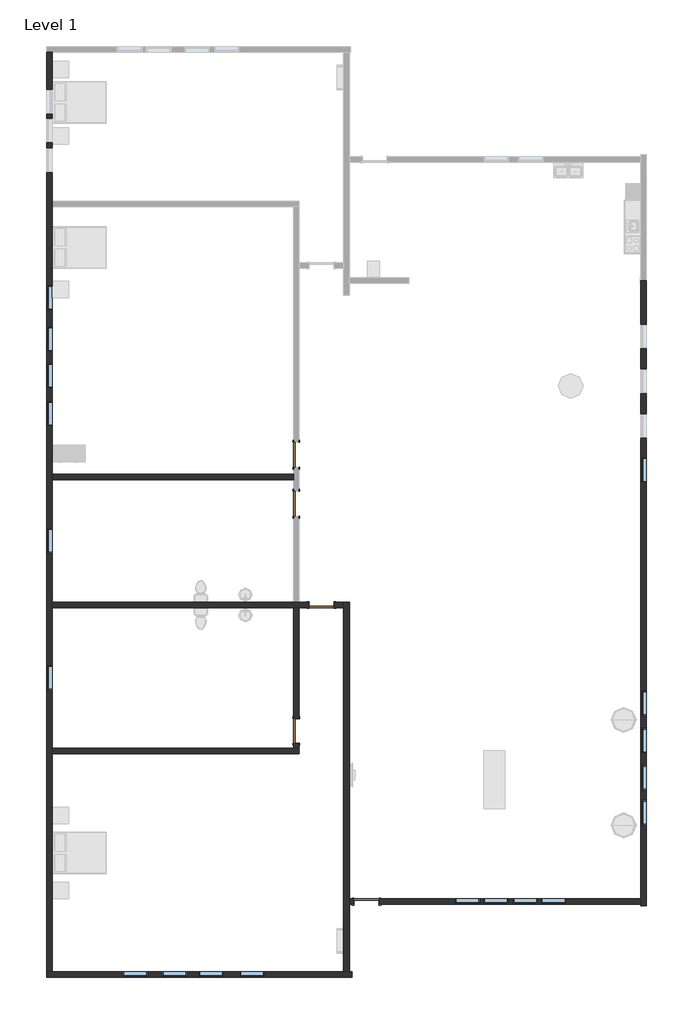
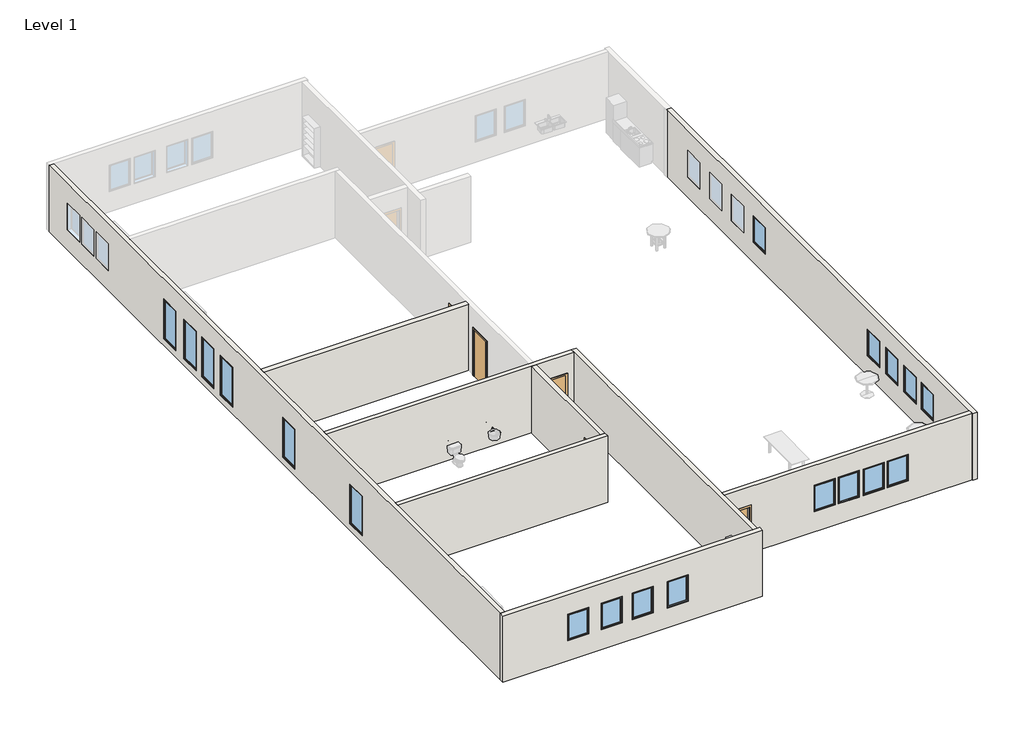
# One storey, part 1 of 2: 19 windows, 9 walls, 5 doors.
"""IFC4 building model written with IfcOpenShell, lengths in millimetres."""

from ifc_helpers import new_model, si_unit, frame, origin, origin_with_axes, place, context, project, spatial, polyline, outline, extrude, faceted_brep, transform, mapped, element, save
from components import door_54dd4da4, door_719f80de, window_e2841890, window_9a779fa2

model = new_model("IFC4")

# Units and contexts
model_context = context("Model", 3, world=origin())
ifc_project = project(units=[si_unit("LENGTHUNIT", "METRE", prefix="MILLI")], contexts=[model_context])

# Site, building, storey
site = spatial("IfcSite", under=ifc_project)
building = spatial("IfcBuilding", under=site)
storey = spatial("IfcBuildingStorey", under=building, Name="Level 1", Elevation=0.0)

# Doors
placement = place(None, origin())
door_shape = door_54dd4da4(model_context)
element("IfcDoor", 1, ObjectType="Single-Flush : 36\" x 84\"", at=placement, inside=storey, context=model_context, shape_type="MappedRepresentation", body=[
    mapped(door_shape, transform((-5497.7112155, -2495.646371, 0.0), x_axis=(0.0, 1.0, 0.0), y_axis=(-1.0, 0.0, 0.0), z_axis=(0.0, 0.0, 1.0))),
])
door_2_shape = door_719f80de(model_context)
element("IfcDoor", 2, ObjectType="Single-Flush : 36\" x 84\"", at=placement, inside=storey, context=model_context, shape_type="MappedRepresentation", body=[
    mapped(door_2_shape, transform((-4570.6112155, -6229.446371, 0.0), x_axis=(1.0, 0.0, 0.0), y_axis=(0.0, 1.0, 0.0), z_axis=(0.0, 0.0, 1.0))),
])
element("IfcDoor", 3, ObjectType="Single-Flush : 36\" x 84\"", at=placement, inside=storey, context=model_context, shape_type="MappedRepresentation", body=[
    mapped(door_2_shape, transform((-5497.7112155, -10877.646371, 0.0), x_axis=(0.0, -1.0, 0.0), y_axis=(1.0, 0.0, 0.0), z_axis=(0.0, 0.0, 1.0))),
])
element("IfcDoor", 4, ObjectType="Single-Flush : 36\" x 84\"", at=placement, inside=storey, context=model_context, shape_type="MappedRepresentation", body=[
    mapped(door_2_shape, transform((-2906.9112155, -17176.846371, 0.0), x_axis=(-1.0, 0.0, 0.0), y_axis=(0.0, -1.0, 0.0), z_axis=(0.0, 0.0, 1.0))),
])
element("IfcDoor", 5, ObjectType="Single-Flush : 36\" x 84\"", at=placement, inside=storey, context=model_context, shape_type="MappedRepresentation", body=[
    mapped(door_2_shape, transform((-5497.7112155, -692.246371, 0.0), x_axis=(0.0, -1.0, 0.0), y_axis=(1.0, 0.0, 0.0), z_axis=(0.0, 0.0, 1.0))),
])

# Walls
element("IfcWall", 6, ObjectType="Generic - 8\"", at=placement, inside=storey, context=model_context, shape_type="Brep", body=[
    faceted_brep([(-14514.7112155, -19767.646371, 0.0), (-14514.7112155, -11715.846371, 0.0), (-14514.7112155, -11512.646371, 0.0), (-14514.7112155, -6331.046371, 0.0), (-14514.7112155, -6127.846371, 0.0), (-14514.7112155, -1606.646371, 0.0), (-14514.7112155, -1403.446371, 0.0), (-14514.7112155, 8451.753629, 0.0), (-14514.7112155, 8654.953629, 0.0), (-14514.7112155, 14166.753629, 0.0), (-14514.7112155, 14166.753629, 3048.0), (-14514.7112155, 8654.953629, 3048.0), (-14514.7112155, 8451.753629, 3048.0), (-14514.7112155, -1403.446371, 3048.0), (-14514.7112155, -1606.646371, 3048.0), (-14514.7112155, -6127.846371, 3048.0), (-14514.7112155, -6331.046371, 3048.0), (-14514.7112155, -11512.646371, 3048.0), (-14514.7112155, -11715.846371, 3048.0), (-14514.7112155, -19767.646371, 3048.0), (-14514.7112155, 11880.753629, 2133.6), (-14514.7112155, 12795.153629, 2133.6), (-14514.7112155, 12795.153629, 914.4), (-14514.7112155, 11880.753629, 914.4), (-14514.7112155, 11728.353629, 2133.6), (-14514.7112155, 11728.353629, 914.4), (-14514.7112155, 10813.953629, 914.4), (-14514.7112155, 10813.953629, 2133.6), (-14514.7112155, 10636.153629, 2133.6), (-14514.7112155, 10636.153629, 914.4), (-14514.7112155, 9721.753629, 914.4), (-14514.7112155, 9721.753629, 2133.6), (-14514.7112155, -8464.646371, 2133.6), (-14514.7112155, -8464.646371, 304.8), (-14514.7112155, -9379.046371, 304.8), (-14514.7112155, -9379.046371, 2133.6), (-14514.7112155, -3410.046371, 2133.6), (-14514.7112155, -3410.046371, 304.8), (-14514.7112155, -4324.446371, 304.8), (-14514.7112155, -4324.446371, 2133.6), (-14514.7112155, 1288.953629, 2133.6), (-14514.7112155, 1288.953629, 304.8), (-14514.7112155, 374.553629, 304.8), (-14514.7112155, 374.553629, 2133.6), (-14514.7112155, 2685.953629, 2133.6), (-14514.7112155, 2685.953629, 304.8), (-14514.7112155, 1771.553629, 304.8), (-14514.7112155, 1771.553629, 2133.6), (-14514.7112155, 4032.153629, 2133.6), (-14514.7112155, 4032.153629, 304.8), (-14514.7112155, 3117.753629, 304.8), (-14514.7112155, 3117.753629, 2133.6), (-14514.7112155, 5556.153629, 2133.6), (-14514.7112155, 5556.153629, 304.8), (-14514.7112155, 4641.753629, 304.8), (-14514.7112155, 4641.753629, 2133.6), (-14717.9112155, -19767.646371, 0.0), (-14717.9112155, -19767.646371, 3048.0), (-14717.9112155, 14166.753629, 3048.0), (-14717.9112155, 14166.753629, 0.0), (-14717.9112155, 11880.753629, 2133.6), (-14717.9112155, 11880.753629, 914.4), (-14717.9112155, 12795.153629, 914.4), (-14717.9112155, 12795.153629, 2133.6), (-14717.9112155, 11728.353629, 2133.6), (-14717.9112155, 10813.953629, 2133.6), (-14717.9112155, 10813.953629, 914.4), (-14717.9112155, 11728.353629, 914.4), (-14717.9112155, 10636.153629, 2133.6), (-14717.9112155, 9721.753629, 2133.6), (-14717.9112155, 9721.753629, 914.4), (-14717.9112155, 10636.153629, 914.4), (-14717.9112155, -8464.646371, 2133.6), (-14717.9112155, -9379.046371, 2133.6), (-14717.9112155, -9379.046371, 304.8), (-14717.9112155, -8464.646371, 304.8), (-14717.9112155, -3410.046371, 2133.6), (-14717.9112155, -4324.446371, 2133.6), (-14717.9112155, -4324.446371, 304.8), (-14717.9112155, -3410.046371, 304.8), (-14717.9112155, 1288.953629, 2133.6), (-14717.9112155, 374.553629, 2133.6), (-14717.9112155, 374.553629, 304.8), (-14717.9112155, 1288.953629, 304.8), (-14717.9112155, 2685.953629, 2133.6), (-14717.9112155, 1771.553629, 2133.6), (-14717.9112155, 1771.553629, 304.8), (-14717.9112155, 2685.953629, 304.8), (-14717.9112155, 4032.153629, 2133.6), (-14717.9112155, 3117.753629, 2133.6), (-14717.9112155, 3117.753629, 304.8), (-14717.9112155, 4032.153629, 304.8), (-14717.9112155, 5556.153629, 2133.6), (-14717.9112155, 4641.753629, 2133.6), (-14717.9112155, 4641.753629, 304.8), (-14717.9112155, 5556.153629, 304.8)], [[[0, 1, 2, 3, 4, 5, 6, 7, 8, 9, 10, 11, 12, 13, 14, 15, 16, 17, 18, 19], [20, 21, 22, 23], [24, 25, 26, 27], [28, 29, 30, 31], [32, 33, 34, 35], [36, 37, 38, 39], [40, 41, 42, 43], [44, 45, 46, 47], [48, 49, 50, 51], [52, 53, 54, 55]], [[56, 57, 58, 59], [60, 61, 62, 63], [64, 65, 66, 67], [68, 69, 70, 71], [72, 73, 74, 75], [76, 77, 78, 79], [80, 81, 82, 83], [84, 85, 86, 87], [88, 89, 90, 91], [92, 93, 94, 95]], [[9, 8, 7, 6, 5, 4, 3, 2, 1, 0, 56, 59]], [[19, 18, 17, 16, 15, 14, 13, 12, 11, 10, 58, 57]], [[10, 9, 59, 58]], [[0, 19, 57, 56]], [[61, 60, 20, 23]], [[62, 61, 23, 22]], [[63, 62, 22, 21]], [[60, 63, 21, 20]], [[25, 24, 64, 67]], [[26, 25, 67, 66]], [[27, 26, 66, 65]], [[24, 27, 65, 64]], [[29, 28, 68, 71]], [[30, 29, 71, 70]], [[31, 30, 70, 69]], [[28, 31, 69, 68]], [[33, 32, 72, 75]], [[34, 33, 75, 74]], [[35, 34, 74, 73]], [[32, 35, 73, 72]], [[37, 36, 76, 79]], [[38, 37, 79, 78]], [[39, 38, 78, 77]], [[36, 39, 77, 76]], [[41, 40, 80, 83]], [[42, 41, 83, 82]], [[43, 42, 82, 81]], [[40, 43, 81, 80]], [[45, 44, 84, 87]], [[46, 45, 87, 86]], [[47, 46, 86, 85]], [[44, 47, 85, 84]], [[49, 48, 88, 91]], [[50, 49, 91, 90]], [[51, 50, 90, 89]], [[48, 51, 89, 88]], [[53, 52, 92, 95]], [[54, 53, 95, 94]], [[55, 54, 94, 93]], [[52, 55, 93, 92]]]),
])
element("IfcWall", 7, ObjectType="Generic - 8\"", at=placement, inside=storey, context=model_context, shape_type="SweptSolid", body=[
    extrude(outline(polyline([(0.0, -3541.9112155), (0.0, -3364.1112155), (2133.6, -3364.1112155), (2133.6, -2449.7112155), (0.0, -2449.7112155), (0.0, 7227.6887845), (3048.0, 7227.6887845), (3048.0, -3541.9112155), (0.0, -3541.9112155)]), holes=[polyline([(2133.6, 369.6887845), (2133.6, 1284.0887845), (914.4, 1284.0887845), (914.4, 369.6887845), (2133.6, 369.6887845)]), polyline([(2133.6, 1411.0887845), (2133.6, 2325.4887845), (914.4, 2325.4887845), (914.4, 1411.0887845), (2133.6, 1411.0887845)]), polyline([(2133.6, 2503.2887845), (2133.6, 3417.6887845), (914.4, 3417.6887845), (914.4, 2503.2887845), (2133.6, 2503.2887845)]), polyline([(2133.6, 3544.6887845), (2133.6, 4459.0887845), (914.4, 4459.0887845), (914.4, 3544.6887845), (2133.6, 3544.6887845)])]), frame((0.0, -17278.446371, 0.0), z_axis=(0.0, 1.0, 0.0), x_axis=(0.0, 0.0, 1.0)), (0.0, 0.0, 1.0), 203.2),
])
element("IfcWall", 8, ObjectType="Generic - 8\"", at=placement, inside=storey, context=model_context, shape_type="Brep", body=[
    faceted_brep([(-4113.4112155, -6331.046371, 2133.6), (-4113.4112155, -6331.046371, 0.0), (-3745.1112155, -6331.046371, 0.0), (-3745.1112155, -6331.046371, 3048.0), (-5396.1112155, -6331.046371, 3048.0), (-5599.3112155, -6331.046371, 3048.0), (-14514.7112155, -6331.046371, 3048.0), (-14514.7112155, -6331.046371, 0.0), (-5599.3112155, -6331.046371, 0.0), (-5396.1112155, -6331.046371, 0.0), (-5027.8112155, -6331.046371, 0.0), (-5027.8112155, -6331.046371, 2133.6), (-3745.1112155, -6127.846371, 0.0), (-4113.4112155, -6127.846371, 0.0), (-4113.4112155, -6127.846371, 2133.6), (-5027.8112155, -6127.846371, 2133.6), (-5027.8112155, -6127.846371, 0.0), (-5396.1112155, -6127.846371, 0.0), (-5599.3112155, -6127.846371, 0.0), (-14514.7112155, -6127.846371, 0.0), (-14514.7112155, -6127.846371, 3048.0), (-5599.3112155, -6127.846371, 3048.0), (-5396.1112155, -6127.846371, 3048.0), (-3745.1112155, -6127.846371, 3048.0)], [[[0, 1, 2, 3, 4, 5, 6, 7, 8, 9, 10, 11]], [[12, 13, 14, 15, 16, 17, 18, 19, 20, 21, 22, 23]], [[2, 1, 13, 12]], [[10, 9, 8, 7, 19, 18, 17, 16]], [[6, 5, 4, 3, 23, 22, 21, 20]], [[7, 6, 20, 19]], [[14, 13, 1, 0]], [[15, 14, 0, 11]], [[16, 15, 11, 10]], [[3, 2, 12, 23]]]),
])
element("IfcWall", 9, ObjectType="Generic - 8\"", at=placement, inside=storey, context=model_context, shape_type="SweptSolid", body=[
    extrude(outline(polyline([(-14514.7112155, -1403.446371), (-5599.3112155, -1403.446371), (-5599.3112155, -1606.646371), (-14514.7112155, -1606.646371), (-14514.7112155, -1403.446371)])), origin_with_axes(), (0.0, 0.0, 1.0), 3048.0),
])
element("IfcWall", 10, ObjectType="Generic - 8\"", at=placement, inside=storey, context=model_context, shape_type="Brep", body=[
    faceted_brep([(-14514.7112155, -11715.846371, 0.0), (-5396.1112155, -11715.846371, 0.0), (-5396.1112155, -11715.846371, 3048.0), (-14514.7112155, -11715.846371, 3048.0), (-14514.7112155, -11512.646371, 0.0), (-14514.7112155, -11512.646371, 3048.0), (-5599.3112155, -11512.646371, 3048.0), (-5396.1112155, -11512.646371, 3048.0), (-5396.1112155, -11512.646371, 0.0), (-5599.3112155, -11512.646371, 0.0)], [[[0, 1, 2, 3]], [[4, 5, 6, 7, 8, 9]], [[1, 0, 4, 9, 8]], [[3, 2, 7, 6, 5]], [[0, 3, 5, 4]], [[2, 1, 8, 7]]]),
])
element("IfcWall", 11, ObjectType="Generic - 8\"", at=placement, inside=storey, context=model_context, shape_type="Brep", body=[
    faceted_brep([(-3745.1112155, -6127.846371, 0.0), (-3745.1112155, -6331.046371, 0.0), (-3745.1112155, -19767.646371, 0.0), (-3745.1112155, -19767.646371, 3048.0), (-3745.1112155, -6331.046371, 3048.0), (-3745.1112155, -6127.846371, 3048.0), (-3541.9112155, -6127.846371, 0.0), (-3541.9112155, -6127.846371, 3048.0), (-3541.9112155, -17075.246371, 3048.0), (-3541.9112155, -17278.446371, 3048.0), (-3541.9112155, -19767.646371, 3048.0), (-3541.9112155, -19767.646371, 0.0), (-3541.9112155, -17278.446371, 0.0), (-3541.9112155, -17075.246371, 0.0)], [[[0, 1, 2, 3, 4, 5]], [[6, 7, 8, 9, 10, 11, 12, 13]], [[2, 1, 0, 6, 13, 12, 11]], [[5, 4, 3, 10, 9, 8, 7]], [[3, 2, 11, 10]], [[0, 5, 7, 6]]]),
])
element("IfcWall", 12, ObjectType="Generic - 8\"", at=placement, inside=storey, context=model_context, shape_type="SweptSolid", body=[
    extrude(outline(polyline([(-11334.846371, 2133.6), (-11334.846371, 0.0), (-11512.646371, 0.0), (-11512.646371, 3048.0), (-6331.046371, 3048.0), (-6331.046371, 0.0), (-10420.446371, 0.0), (-10420.446371, 2133.6), (-11334.846371, 2133.6)])), frame((-5599.3112155, 0.0, 0.0), z_axis=(1.0, 0.0, 0.0), x_axis=(0.0, 1.0, 0.0)), (0.0, 0.0, 1.0), 203.2),
])
element("IfcWall", 13, ObjectType="Generic - 8\"", at=placement, inside=storey, context=model_context, shape_type="Brep", body=[
    faceted_brep([(7227.6887845, 5733.953629, 0.0), (7227.6887845, 5632.353629, 0.0), (7227.6887845, -17075.246371, 0.0), (7227.6887845, -17278.446371, 0.0), (7227.6887845, -17329.246371, 0.0), (7227.6887845, -17329.246371, 3048.0), (7227.6887845, -17278.446371, 3048.0), (7227.6887845, -17075.246371, 3048.0), (7227.6887845, 5632.353629, 3048.0), (7227.6887845, 5733.953629, 3048.0), (7227.6887845, 4133.753629, 2133.6), (7227.6887845, 3219.353629, 2133.6), (7227.6887845, 3219.353629, 914.4), (7227.6887845, 4133.753629, 914.4), (7227.6887845, 2482.753629, 2133.6), (7227.6887845, 1568.353629, 2133.6), (7227.6887845, 1568.353629, 914.4), (7227.6887845, 2482.753629, 914.4), (7227.6887845, 831.753629, 2133.6), (7227.6887845, -82.646371, 2133.6), (7227.6887845, -82.646371, 914.4), (7227.6887845, 831.753629, 914.4), (7227.6887845, -793.846371, 2133.6), (7227.6887845, -1708.246371, 2133.6), (7227.6887845, -1708.246371, 914.4), (7227.6887845, -793.846371, 914.4), (7227.6887845, -13443.046371, 2133.6), (7227.6887845, -14357.446371, 2133.6), (7227.6887845, -14357.446371, 914.4), (7227.6887845, -13443.046371, 914.4), (7227.6887845, -12147.646371, 2133.6), (7227.6887845, -13062.046371, 2133.6), (7227.6887845, -13062.046371, 914.4), (7227.6887845, -12147.646371, 914.4), (7227.6887845, -10776.046371, 2133.6), (7227.6887845, -11690.446371, 2133.6), (7227.6887845, -11690.446371, 914.4), (7227.6887845, -10776.046371, 914.4), (7227.6887845, -9404.446371, 2133.6), (7227.6887845, -10318.846371, 2133.6), (7227.6887845, -10318.846371, 914.4), (7227.6887845, -9404.446371, 914.4), (7430.8887845, 5733.953629, 0.0), (7430.8887845, 5733.953629, 3048.0), (7430.8887845, -17329.246371, 3048.0), (7430.8887845, -17329.246371, 0.0), (7430.8887845, 4133.753629, 2133.6), (7430.8887845, 4133.753629, 914.4), (7430.8887845, 3219.353629, 914.4), (7430.8887845, 3219.353629, 2133.6), (7430.8887845, 2482.753629, 2133.6), (7430.8887845, 2482.753629, 914.4), (7430.8887845, 1568.353629, 914.4), (7430.8887845, 1568.353629, 2133.6), (7430.8887845, 831.753629, 2133.6), (7430.8887845, 831.753629, 914.4), (7430.8887845, -82.646371, 914.4), (7430.8887845, -82.646371, 2133.6), (7430.8887845, -793.846371, 2133.6), (7430.8887845, -793.846371, 914.4), (7430.8887845, -1708.246371, 914.4), (7430.8887845, -1708.246371, 2133.6), (7430.8887845, -13443.046371, 2133.6), (7430.8887845, -13443.046371, 914.4), (7430.8887845, -14357.446371, 914.4), (7430.8887845, -14357.446371, 2133.6), (7430.8887845, -12147.646371, 2133.6), (7430.8887845, -12147.646371, 914.4), (7430.8887845, -13062.046371, 914.4), (7430.8887845, -13062.046371, 2133.6), (7430.8887845, -10776.046371, 2133.6), (7430.8887845, -10776.046371, 914.4), (7430.8887845, -11690.446371, 914.4), (7430.8887845, -11690.446371, 2133.6), (7430.8887845, -9404.446371, 2133.6), (7430.8887845, -9404.446371, 914.4), (7430.8887845, -10318.846371, 914.4), (7430.8887845, -10318.846371, 2133.6)], [[[0, 1, 2, 3, 4, 5, 6, 7, 8, 9], [10, 11, 12, 13], [14, 15, 16, 17], [18, 19, 20, 21], [22, 23, 24, 25], [26, 27, 28, 29], [30, 31, 32, 33], [34, 35, 36, 37], [38, 39, 40, 41]], [[42, 43, 44, 45], [46, 47, 48, 49], [50, 51, 52, 53], [54, 55, 56, 57], [58, 59, 60, 61], [62, 63, 64, 65], [66, 67, 68, 69], [70, 71, 72, 73], [74, 75, 76, 77]], [[4, 3, 2, 1, 0, 42, 45]], [[5, 4, 45, 44]], [[9, 8, 7, 6, 5, 44, 43]], [[0, 9, 43, 42]], [[47, 46, 10, 13]], [[48, 47, 13, 12]], [[49, 48, 12, 11]], [[46, 49, 11, 10]], [[51, 50, 14, 17]], [[52, 51, 17, 16]], [[53, 52, 16, 15]], [[50, 53, 15, 14]], [[55, 54, 18, 21]], [[56, 55, 21, 20]], [[57, 56, 20, 19]], [[54, 57, 19, 18]], [[59, 58, 22, 25]], [[60, 59, 25, 24]], [[61, 60, 24, 23]], [[58, 61, 23, 22]], [[63, 62, 26, 29]], [[64, 63, 29, 28]], [[65, 64, 28, 27]], [[62, 65, 27, 26]], [[67, 66, 30, 33]], [[68, 67, 33, 32]], [[69, 68, 32, 31]], [[66, 69, 31, 30]], [[71, 70, 34, 37]], [[72, 71, 37, 36]], [[73, 72, 36, 35]], [[70, 73, 35, 34]], [[75, 74, 38, 41]], [[76, 75, 41, 40]], [[77, 76, 40, 39]], [[74, 77, 39, 38]]]),
])
element("IfcWall", 14, ObjectType="Generic - 8\"", at=placement, inside=storey, context=model_context, shape_type="Brep", body=[
    faceted_brep([(-3440.3112155, -19767.646371, 0.0), (-3541.9112155, -19767.646371, 0.0), (-3745.1112155, -19767.646371, 0.0), (-14514.7112155, -19767.646371, 0.0), (-14717.9112155, -19767.646371, 0.0), (-14717.9112155, -19767.646371, 3048.0), (-14514.7112155, -19767.646371, 3048.0), (-3745.1112155, -19767.646371, 3048.0), (-3541.9112155, -19767.646371, 3048.0), (-3440.3112155, -19767.646371, 3048.0), (-7580.5112155, -19767.646371, 2133.6), (-7580.5112155, -19767.646371, 914.4), (-6666.1112155, -19767.646371, 914.4), (-6666.1112155, -19767.646371, 2133.6), (-9104.5112155, -19767.646371, 2133.6), (-9104.5112155, -19767.646371, 914.4), (-8190.1112155, -19767.646371, 914.4), (-8190.1112155, -19767.646371, 2133.6), (-10450.7112155, -19767.646371, 2133.6), (-10450.7112155, -19767.646371, 914.4), (-9536.3112155, -19767.646371, 914.4), (-9536.3112155, -19767.646371, 2133.6), (-11898.5112155, -19767.646371, 2133.6), (-11898.5112155, -19767.646371, 914.4), (-10984.1112155, -19767.646371, 914.4), (-10984.1112155, -19767.646371, 2133.6), (-3440.3112155, -19970.846371, 0.0), (-3440.3112155, -19970.846371, 3048.0), (-14717.9112155, -19970.846371, 3048.0), (-14717.9112155, -19970.846371, 0.0), (-7580.5112155, -19970.846371, 2133.6), (-6666.1112155, -19970.846371, 2133.6), (-6666.1112155, -19970.846371, 914.4), (-7580.5112155, -19970.846371, 914.4), (-9104.5112155, -19970.846371, 2133.6), (-8190.1112155, -19970.846371, 2133.6), (-8190.1112155, -19970.846371, 914.4), (-9104.5112155, -19970.846371, 914.4), (-10450.7112155, -19970.846371, 2133.6), (-9536.3112155, -19970.846371, 2133.6), (-9536.3112155, -19970.846371, 914.4), (-10450.7112155, -19970.846371, 914.4), (-11898.5112155, -19970.846371, 2133.6), (-10984.1112155, -19970.846371, 2133.6), (-10984.1112155, -19970.846371, 914.4), (-11898.5112155, -19970.846371, 914.4)], [[[0, 1, 2, 3, 4, 5, 6, 7, 8, 9], [10, 11, 12, 13], [14, 15, 16, 17], [18, 19, 20, 21], [22, 23, 24, 25]], [[26, 27, 28, 29], [30, 31, 32, 33], [34, 35, 36, 37], [38, 39, 40, 41], [42, 43, 44, 45]], [[4, 3, 2, 1, 0, 26, 29]], [[9, 8, 7, 6, 5, 28, 27]], [[0, 9, 27, 26]], [[5, 4, 29, 28]], [[10, 13, 31, 30]], [[13, 12, 32, 31]], [[12, 11, 33, 32]], [[11, 10, 30, 33]], [[14, 17, 35, 34]], [[17, 16, 36, 35]], [[16, 15, 37, 36]], [[15, 14, 34, 37]], [[18, 21, 39, 38]], [[21, 20, 40, 39]], [[20, 19, 41, 40]], [[19, 18, 38, 41]], [[22, 25, 43, 42]], [[25, 24, 44, 43]], [[24, 23, 45, 44]], [[23, 22, 42, 45]]]),
])

# Windows
window_shape = window_e2841890(model_context)
element("IfcWindow", 15, ObjectType="Fixed : 36\" x 48\"", at=placement, inside=storey, context=model_context, shape_type="MappedRepresentation", body=[
    mapped(window_shape, transform((7329.2887845, -1212.946371, 0.0), x_axis=(0.0, 1.0, 0.0), y_axis=(-1.0, 0.0, 0.0), z_axis=(0.0, 0.0, 1.0))),
])
element("IfcWindow", 16, ObjectType="Fixed : 36\" x 48\"", at=placement, inside=storey, context=model_context, shape_type="MappedRepresentation", body=[
    mapped(window_shape, transform((7329.2887845, -13862.146371, 0.0), x_axis=(0.0, 1.0, 0.0), y_axis=(-1.0, 0.0, 0.0), z_axis=(0.0, 0.0, 1.0))),
])
element("IfcWindow", 17, ObjectType="Fixed : 36\" x 48\"", at=placement, inside=storey, context=model_context, shape_type="MappedRepresentation", body=[
    mapped(window_shape, transform((7329.2887845, -12566.746371, 0.0), x_axis=(0.0, 1.0, 0.0), y_axis=(-1.0, 0.0, 0.0), z_axis=(0.0, 0.0, 1.0))),
])
element("IfcWindow", 18, ObjectType="Fixed : 36\" x 48\"", at=placement, inside=storey, context=model_context, shape_type="MappedRepresentation", body=[
    mapped(window_shape, transform((7329.2887845, -11195.146371, 0.0), x_axis=(0.0, 1.0, 0.0), y_axis=(-1.0, 0.0, 0.0), z_axis=(0.0, 0.0, 1.0))),
])
element("IfcWindow", 19, ObjectType="Fixed : 36\" x 48\"", at=placement, inside=storey, context=model_context, shape_type="MappedRepresentation", body=[
    mapped(window_shape, transform((7329.2887845, -9823.546371, 0.0), x_axis=(0.0, 1.0, 0.0), y_axis=(-1.0, 0.0, 0.0), z_axis=(0.0, 0.0, 1.0))),
])
element("IfcWindow", 20, ObjectType="Fixed : 36\" x 48\"", at=placement, inside=storey, context=model_context, shape_type="MappedRepresentation", body=[
    mapped(window_shape, transform((788.7887845, -17176.846371, 0.0), x_axis=(-1.0, 0.0, 0.0), y_axis=(0.0, -1.0, 0.0), z_axis=(0.0, 0.0, 1.0))),
])
element("IfcWindow", 21, ObjectType="Fixed : 36\" x 48\"", at=placement, inside=storey, context=model_context, shape_type="MappedRepresentation", body=[
    mapped(window_shape, transform((1830.1887845, -17176.846371, 0.0), x_axis=(-1.0, 0.0, 0.0), y_axis=(0.0, -1.0, 0.0), z_axis=(0.0, 0.0, 1.0))),
])
element("IfcWindow", 22, ObjectType="Fixed : 36\" x 48\"", at=placement, inside=storey, context=model_context, shape_type="MappedRepresentation", body=[
    mapped(window_shape, transform((2922.3887845, -17176.846371, 0.0), x_axis=(-1.0, 0.0, 0.0), y_axis=(0.0, -1.0, 0.0), z_axis=(0.0, 0.0, 1.0))),
])
element("IfcWindow", 23, ObjectType="Fixed : 36\" x 48\"", at=placement, inside=storey, context=model_context, shape_type="MappedRepresentation", body=[
    mapped(window_shape, transform((3963.7887845, -17176.846371, 0.0), x_axis=(-1.0, 0.0, 0.0), y_axis=(0.0, -1.0, 0.0), z_axis=(0.0, 0.0, 1.0))),
])
element("IfcWindow", 24, ObjectType="Fixed : 36\" x 48\"", at=placement, inside=storey, context=model_context, shape_type="MappedRepresentation", body=[
    mapped(window_shape, transform((-7161.4112155, -19869.246371, 0.0), x_axis=(-1.0, 0.0, 0.0), y_axis=(0.0, -1.0, 0.0), z_axis=(0.0, 0.0, 1.0))),
])
element("IfcWindow", 25, ObjectType="Fixed : 36\" x 48\"", at=placement, inside=storey, context=model_context, shape_type="MappedRepresentation", body=[
    mapped(window_shape, transform((-8685.4112155, -19869.246371, 0.0), x_axis=(-1.0, 0.0, 0.0), y_axis=(0.0, -1.0, 0.0), z_axis=(0.0, 0.0, 1.0))),
])
element("IfcWindow", 26, ObjectType="Fixed : 36\" x 48\"", at=placement, inside=storey, context=model_context, shape_type="MappedRepresentation", body=[
    mapped(window_shape, transform((-10031.6112155, -19869.246371, 0.0), x_axis=(-1.0, 0.0, 0.0), y_axis=(0.0, -1.0, 0.0), z_axis=(0.0, 0.0, 1.0))),
])
element("IfcWindow", 27, ObjectType="Fixed : 36\" x 48\"", at=placement, inside=storey, context=model_context, shape_type="MappedRepresentation", body=[
    mapped(window_shape, transform((-11479.4112155, -19869.246371, 0.0), x_axis=(-1.0, 0.0, 0.0), y_axis=(0.0, -1.0, 0.0), z_axis=(0.0, 0.0, 1.0))),
])
window_2_shape = window_9a779fa2(model_context)
element("IfcWindow", 28, ObjectType="Fixed : 36\" x 72\"", at=placement, inside=storey, context=model_context, shape_type="MappedRepresentation", body=[
    mapped(window_2_shape, transform((-14616.3112155, -8883.746371, 0.0), x_axis=(0.0, 1.0, 0.0), y_axis=(-1.0, 0.0, 0.0), z_axis=(0.0, 0.0, 1.0))),
])
element("IfcWindow", 29, ObjectType="Fixed : 36\" x 72\"", at=placement, inside=storey, context=model_context, shape_type="MappedRepresentation", body=[
    mapped(window_2_shape, transform((-14616.3112155, -3829.146371, 0.0), x_axis=(0.0, 1.0, 0.0), y_axis=(-1.0, 0.0, 0.0), z_axis=(0.0, 0.0, 1.0))),
])
element("IfcWindow", 30, ObjectType="Fixed : 36\" x 72\"", at=placement, inside=storey, context=model_context, shape_type="MappedRepresentation", body=[
    mapped(window_2_shape, transform((-14616.3112155, 869.853629, 0.0), x_axis=(0.0, 1.0, 0.0), y_axis=(-1.0, 0.0, 0.0), z_axis=(0.0, 0.0, 1.0))),
])
element("IfcWindow", 31, ObjectType="Fixed : 36\" x 72\"", at=placement, inside=storey, context=model_context, shape_type="MappedRepresentation", body=[
    mapped(window_2_shape, transform((-14616.3112155, 2266.853629, 0.0), x_axis=(0.0, 1.0, 0.0), y_axis=(-1.0, 0.0, 0.0), z_axis=(0.0, 0.0, 1.0))),
])
element("IfcWindow", 32, ObjectType="Fixed : 36\" x 72\"", at=placement, inside=storey, context=model_context, shape_type="MappedRepresentation", body=[
    mapped(window_2_shape, transform((-14616.3112155, 3613.053629, 0.0), x_axis=(0.0, 1.0, 0.0), y_axis=(-1.0, 0.0, 0.0), z_axis=(0.0, 0.0, 1.0))),
])
element("IfcWindow", 33, ObjectType="Fixed : 36\" x 72\"", at=placement, inside=storey, context=model_context, shape_type="MappedRepresentation", body=[
    mapped(window_2_shape, transform((-14616.3112155, 5137.053629, 0.0), x_axis=(0.0, 1.0, 0.0), y_axis=(-1.0, 0.0, 0.0), z_axis=(0.0, 0.0, 1.0))),
])

save(model, "model.ifc")

# Revit data of these elements
# Type "Single-Flush : 36\" x 84\""
#   Type Mark = "1"
#   Construction Type Id = "MDOOR"
#   Assembly Code = "C1020"
#   Analytic Construction = "Metal"
#   Thickness = 0' - 2"
#   Heat Transfer Coefficient (U) = 0.651978 BTU/(h·ft²·°F)
#   Height = 7' - 0"
#   Trim Projection Ext = 0' - 1"
#   Trim Projection Int = 0' - 1"
#   Trim Width = 0' - 3"
#   Width = 3' - 0"
#   Define Thermal Properties by = 1
#   Door Material = Door - Panel
#   Frame Material = Door - Frame
#   Visual Light Transmittance = 0
#   Solar Heat Gain Coefficient = 0
#   Function = (empty or 0)
#   Wall Closure = (empty or 0)
# Type "Generic - 8\""
#   Assembly Code = "B2010"
#   Layers, outside or top first: 0' - 8" no material (function 1)
# Type "Fixed : 36\" x 48\""
#   Type Mark = "1"
#   Construction Type Id = "GSP4R"
#   Assembly Code = "B2020100"
#   Analytic Construction = "1/8 in Pilkington single glazing"
#   Visual Light Transmittance = 0.9
#   Solar Heat Gain Coefficient = 0.78
#   Heat Transfer Coefficient (U) = 0.6496 BTU/(h·ft²·°F)
#   Height = 4' - 0"
#   Default Sill Height = 3' - 0"
#   Width = 3' - 0"
#   Window Inset = 0' - 0 3/4"
#   Define Thermal Properties by = 1
#   Glass Pane Material = Glass
#   Sash Material = Sash
#   Wall Closure = (empty or 0)
# Type "Fixed : 36\" x 72\""
#   Type Mark = "9"
#   Construction Type Id = "GSP4R"
#   Assembly Code = "B2020100"
#   Analytic Construction = "1/8 in Pilkington single glazing"
#   Visual Light Transmittance = 0.9
#   Solar Heat Gain Coefficient = 0.78
#   Heat Transfer Coefficient (U) = 0.6496 BTU/(h·ft²·°F)
#   Height = 6' - 0"
#   Default Sill Height = 1' - 0"
#   Width = 3' - 0"
#   Window Inset = 0' - 0 3/4"
#   Define Thermal Properties by = 1
#   Glass Pane Material = Glass
#   Sash Material = Sash
#   Wall Closure = (empty or 0)
# Elements 1, 2, 3, 4, 5 (IfcDoor, "Single-Flush : 36\" x 84\"")
#   Phase Created = New Construction
#   Materials on its faces: "Door - Frame", "Door - Panel"
# Elements 6, 7, 8, 9, 10, 11, 12, 13, 14 (IfcWall, "Generic - 8\"")
#   Top Offset = 0' - 0"
#   Base Offset = 0' - 0"
#   Unconnected Height = 10' - 0"
#   wall height = 10' - 0"
#   Phase Created = New Construction
#   Base Constraint = Level 1
#   Materials on its faces: "Default Wall"
# Element 15 (IfcWindow, "Fixed : 36\" x 48\"")
#   Mark = "13"
#   Phase Created = New Construction
#   Materials on its faces: "Sash", "Glass"
# Element 16 (IfcWindow, "Fixed : 36\" x 48\"")
#   Mark = "14"
#   Phase Created = New Construction
#   Materials on its faces: "Sash", "Glass"
# Element 17 (IfcWindow, "Fixed : 36\" x 48\"")
#   Mark = "15"
#   Phase Created = New Construction
#   Materials on its faces: "Sash", "Glass"
# Element 18 (IfcWindow, "Fixed : 36\" x 48\"")
#   Mark = "16"
#   Phase Created = New Construction
#   Materials on its faces: "Sash", "Glass"
# Element 19 (IfcWindow, "Fixed : 36\" x 48\"")
#   Mark = "17"
#   Phase Created = New Construction
#   Materials on its faces: "Sash", "Glass"
# Element 20 (IfcWindow, "Fixed : 36\" x 48\"")
#   Mark = "18"
#   Phase Created = New Construction
#   Materials on its faces: "Sash", "Glass"
# Element 21 (IfcWindow, "Fixed : 36\" x 48\"")
#   Mark = "19"
#   Phase Created = New Construction
#   Materials on its faces: "Sash", "Glass"
# Element 22 (IfcWindow, "Fixed : 36\" x 48\"")
#   Mark = "20"
#   Phase Created = New Construction
#   Materials on its faces: "Sash", "Glass"
# Element 23 (IfcWindow, "Fixed : 36\" x 48\"")
#   Mark = "21"
#   Phase Created = New Construction
#   Materials on its faces: "Sash", "Glass"
# Element 24 (IfcWindow, "Fixed : 36\" x 48\"")
#   Mark = "22"
#   Phase Created = New Construction
#   Materials on its faces: "Sash", "Glass"
# Element 25 (IfcWindow, "Fixed : 36\" x 48\"")
#   Mark = "23"
#   Phase Created = New Construction
#   Materials on its faces: "Sash", "Glass"
# Element 26 (IfcWindow, "Fixed : 36\" x 48\"")
#   Mark = "24"
#   Phase Created = New Construction
#   Materials on its faces: "Sash", "Glass"
# Element 27 (IfcWindow, "Fixed : 36\" x 48\"")
#   Mark = "25"
#   Phase Created = New Construction
#   Materials on its faces: "Sash", "Glass"
# Element 28 (IfcWindow, "Fixed : 36\" x 72\"")
#   Mark = "26"
#   Phase Created = New Construction
#   Materials on its faces: "Sash", "Glass"
# Element 29 (IfcWindow, "Fixed : 36\" x 72\"")
#   Mark = "27"
#   Phase Created = New Construction
#   Materials on its faces: "Sash", "Glass"
# Element 30 (IfcWindow, "Fixed : 36\" x 72\"")
#   Mark = "28"
#   Phase Created = New Construction
#   Materials on its faces: "Sash", "Glass"
# Element 31 (IfcWindow, "Fixed : 36\" x 72\"")
#   Mark = "29"
#   Phase Created = New Construction
#   Materials on its faces: "Sash", "Glass"
# Element 32 (IfcWindow, "Fixed : 36\" x 72\"")
#   Mark = "30"
#   Phase Created = New Construction
#   Materials on its faces: "Sash", "Glass"
# Element 33 (IfcWindow, "Fixed : 36\" x 72\"")
#   Mark = "31"
#   Phase Created = New Construction
#   Materials on its faces: "Sash", "Glass"
# Materials
#   "Door - Panel": class "Wood", colour RGB 210 159 95, transparency 0
#   "Door - Frame": colour RGB 118 70 51, transparency 0
#   "Glass": class "Glass", colour RGB 0 128 192, transparency 0.75, Description = "Soda Lime Glass", Cost = 0
#   "Sash": class "Wood", colour RGB 224 178 126, transparency 0
#   "Default Wall": colour RGB 128 128 128, transparency 0
# Room at (-8819.34, 11368.054) mm, phase "New Construction", upper level "Level 1", upper offset 10' - 0", lower offset 0' - 0"
#   Number = "3"
#   Name = "BED ROOM"
# Room at (-9712.413, 3330.397) mm, phase "New Construction", upper level "Level 1", upper offset 10' - 0", lower offset 0' - 0"
#   Number = "2"
#   Name = "BED ROOM"
# Room at (-10648.14, -3535.102) mm, phase "New Construction", upper level "Level 1", upper offset 10' - 0", lower offset 0' - 0"
#   Number = "2"
# Room at (-10648.14, -8614.454) mm, phase "New Construction", upper level "Level 1", upper offset 10' - 0", lower offset 0' - 0"
#   Number = "1"
# Room at (-8819.34, -15535.77) mm, phase "New Construction", upper level "Level 1", upper offset 10' - 0", lower offset 0' - 0"
#   Number = "1"
#   Name = "BED ROOM"
# Room at (2176.621, -18549.892) mm, phase "New Construction", upper level "Level 1", upper offset 10' - 0", lower offset 0' - 0"
#   Number = "AREA"
#   Name = "PORCH"
# Room at (2176.621, -11684.393) mm, phase "New Construction", upper level "Level 1", upper offset 10' - 0", lower offset 0' - 0"
#   Number = "AREA"
#   Name = "LIVING"
# Room at (2176.621, 3330.397) mm, phase "New Construction", upper level "Level 1", upper offset 10' - 0", lower offset 0' - 0"
#   Number = "8"
#   Name = "Room"
# Room at (2176.621, 8243.537) mm, phase "New Construction", upper level "Level 1", upper offset 10' - 0", lower offset 0' - 0"
#   Number = "AREA"
#   Name = "KITCHEN"
# Room at (1434.806, 12630.209) mm, phase "New Construction", upper level "Level 1", upper offset 10' - 0", lower offset 0' - 0"
#   Number = "AREA"
#   Name = "DIRTY KITCHEN"
# Room at (1754.745, 2068.241) mm, phase "New Construction", upper level "Level 1", upper offset 10' - 0", lower offset 0' - 0"
#   Number = "AREA"
